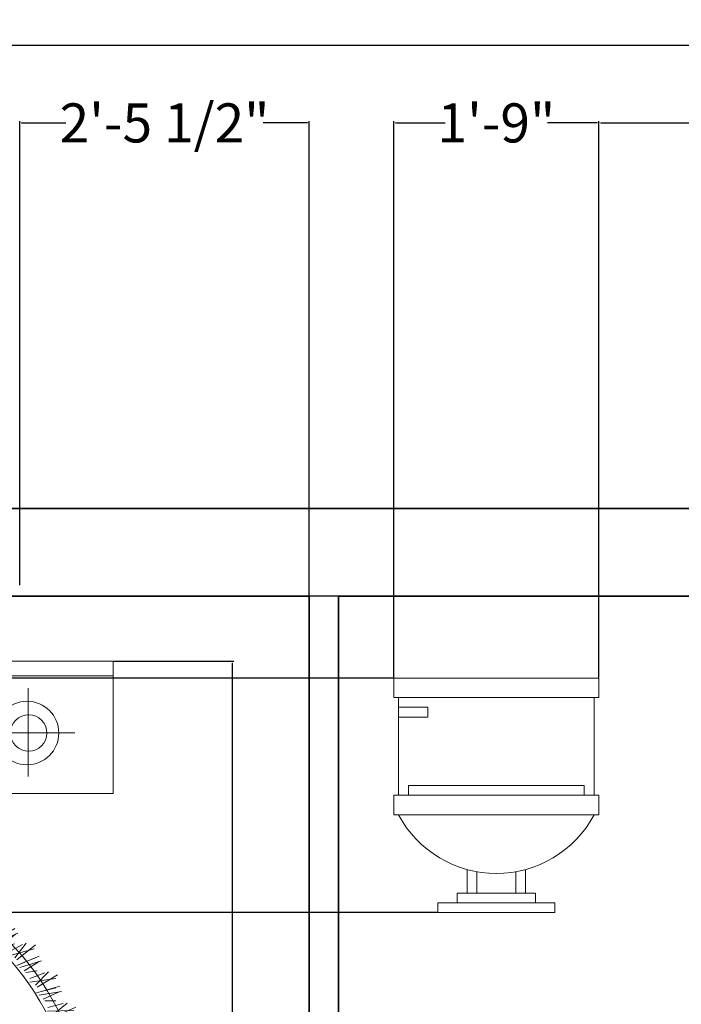
# Model space of a CAD drawing. Units: inches. Extents: x 311 to 754, y 60 to 497.
# Tile 5 of 11: x 462 to 530, y 396 to 497. Entities that reach past the tile are written whole.
import ezdxf

# ---------------------------------------------------------------- set-up
doc = ezdxf.new("R2010")
doc.units = ezdxf.units.IN
doc.header["$MEASUREMENT"] = 0
for name, color, linetype, lineweight in [('A-ANNO-DIMS', 2, 'Continuous', 18), ('A-FLOR-FIXT', 9, 'Continuous', 18), ('A-WALL', 7, 'Continuous', 35), ('beds', 70, 'Continuous', 13)]:
    doc.layers.add(name, color=color, linetype=linetype, lineweight=lineweight)
doc.styles.get("Standard").update_dxf_attribs({"font": 'arial.ttf'})
doc.dimstyles.get("Standard").update_dxf_attribs({"dimtxt": 4, "dimasz": 0.18, "dimexe": 0.18, "dimexo": 0.0625, "dimgap": 0.09, "dimtad": 0, "dimtih": 1, "dimtoh": 1, "dimdec": 0, "dimrnd": 6, "dimzin": 0, "dimdsep": 46, "dimlunit": 3, "dimtxsty": 'Standard', "dimcen": 0.09, "dimadec": 0, "dimazin": 0, "dimtfac": 1, "dimtdec": 0, "dimtofl": 0, "dimtmove": 0, "dimatfit": 3, "dimfxl": 1, "dimtolj": 1, "dimtzin": 0, "dimarcsym": 0})

# ---------------------------------------------------------------- blocks, each defined once
blk = doc.blocks.new('A$C57792D97')
for p, q in [((0.6, 2.6235), (0, 2.6235)), ((0, 2.6235), (0, 2.1735)), ((2.1, 2.6235), (0.6, 2.6235)), ((0.6, 2.6235), (0.6, 0.6235)), ((0.6, 0.6235), (0.6, 2.6235)), ((0.6, 2.1735), (0.6, 2.6235)), ((2.1, 0.6235), (2.1, 2.6235)), ((2.7, 2.6235), (2.1, 2.6235)), ((2.1, 2.6235), (2.1, 2.1735)), ((2.7, 2.1735), (2.7, 2.6235)), ((0.6, 2.5735), (0, 2.5735)), ((2.1, 2.5735), (0.6, 2.5735)), ((2.7, 2.5735), (2.1, 2.5735)), ((2.4103, 2.2312), (2.4103, 2.5317)), ((2.2593, 2.3802), (2.5698, 2.3802)), ((1.5491, 2.1955), (1.5516, 2.1955)), ((0, 2.1735), (0.6, 2.1735)), ((0.6, 2.1518), (0.8661, 2.1518)), ((2.1, 2.1735), (2.7, 2.1735)), ((0.6, 1.9518), (1.4767, 1.9518)), ((0.63, 0.6535), (0.63, 1.9518)), ((0.9906, 1.8942), (0.9508, 1.934)), ((1.4149, 1.8942), (1.3751, 1.934)), ((0.9906, 1.8942), (0.9344, 1.8942)), ((0.9906, 1.8942), (0.9508, 1.8544)), ((1.4149, 1.8942), (1.3586, 1.8942)), ((1.4149, 1.8942), (1.3751, 1.8544)), ((2.142, 1.8959), (2.1018, 1.8254)), ((2.1679, 1.8652), (2.1088, 1.8077)), ((2.1584, 1.8544), (2.1201, 1.8188)), ((2.1812, 1.8524), (2.1207, 1.8046)), ((2.1749, 1.8475), (2.1394, 1.7993)), ((2.1799, 1.8155), (2.1465, 1.7971)), ((2.2066, 1.8191), (2.1664, 1.7827)), ((2.249, 1.8154), (2.1711, 1.7709)), ((2.2173, 1.8274), (2.1931, 1.7688)), ((2.2496, 1.8292), (2.2008, 1.7642)), ((2.07, 1.7793), (2.07, 0.6535)), ((2.2713, 1.7954), (2.2055, 1.7458)), ((2.283, 1.7811), (2.2169, 1.7413)), ((2.2607, 1.7859), (2.2181, 1.7554)), ((2.2761, 1.777), (2.2348, 1.7337)), ((2.277, 1.7446), (2.2416, 1.7306)), ((2.304, 1.7449), (2.2596, 1.7138)), ((2.3157, 1.7518), (2.2843, 1.6966)), ((2.3479, 1.7495), (2.2914, 1.6911)), ((0.7785, 1.6821), (0.7387, 1.7219)), ((1.2027, 1.6821), (1.163, 1.7219)), ((1.627, 1.6821), (1.5872, 1.7219)), ((2.0513, 1.6821), (2.0115, 1.7219)), ((2.3456, 1.7359), (2.2627, 1.7015)), ((2.3653, 1.7133), (2.2937, 1.6723)), ((0.7785, 1.6821), (0.7222, 1.6821)), ((0.7785, 1.6821), (0.7387, 1.6423)), ((1.2027, 1.6821), (1.1465, 1.6821)), ((1.2027, 1.6821), (1.163, 1.6423)), ((1.627, 1.6821), (1.5708, 1.6821)), ((1.627, 1.6821), (1.5872, 1.6423)), ((2.0513, 1.6821), (1.995, 1.6821)), ((2.0513, 1.6821), (2.0115, 1.6423)), ((2.3751, 1.6976), (2.3045, 1.6664)), ((2.3535, 1.7051), (2.3075, 1.6802)), ((2.3677, 1.6944), (2.3213, 1.6565)), ((2.3645, 1.6621), (2.3277, 1.6526)), ((2.3913, 1.659), (2.3434, 1.6337)), ((2.4314, 1.6449), (2.3449, 1.6211)), ((2.4038, 1.6644), (2.3657, 1.6136)), ((2.4355, 1.6581), (2.372, 1.6073)), ((2.4482, 1.62), (2.372, 1.5882)), ((2.4354, 1.6134), (2.3867, 1.5944)), ((2.2754, 1.598), (2.2534, 1.5939)), ((2.2736, 1.5771), (2.2535, 1.594)), ((2.2736, 1.5771), (2.2754, 1.598)), ((2.4559, 1.6032), (2.382, 1.581)), ((2.4482, 1.6009), (2.3974, 1.5692)), ((2.3123, 1.541), (2.2911, 1.5481)), ((2.3006, 1.5236), (2.2912, 1.5481)), ((2.441, 1.5693), (2.4032, 1.5645)), ((2.4672, 1.5629), (2.4164, 1.5438)), ((2.5052, 1.5438), (2.4164, 1.5311)), ((2.4802, 1.5667), (2.4361, 1.5211)), ((2.5109, 1.5564), (2.4416, 1.514)), ((0.9906, 1.47), (0.9508, 1.5097)), ((1.4149, 1.47), (1.3751, 1.5097)), ((1.8391, 1.47), (1.7994, 1.5097)), ((2.3006, 1.5236), (2.3123, 1.541)), ((2.5187, 1.517), (2.4392, 1.4951)), ((2.5052, 1.5121), (2.4545, 1.4994)), ((2.5243, 1.4994), (2.4482, 1.4867)), ((2.5163, 1.4981), (2.462, 1.473)), ((0.9906, 1.47), (0.9344, 1.47)), ((0.9906, 1.47), (0.9508, 1.4302)), ((1.4149, 1.47), (1.3586, 1.47)), ((1.4149, 1.47), (1.3751, 1.4302)), ((1.8391, 1.47), (1.7829, 1.47)), ((1.8391, 1.47), (1.7994, 1.4302)), ((2.5052, 1.4677), (2.4672, 1.4677)), ((2.5304, 1.458), (2.4777, 1.4454)), ((2.5438, 1.4601), (2.4943, 1.4204)), ((2.573, 1.4461), (2.4989, 1.4127)), ((2.5658, 1.4343), (2.4761, 1.4328)), ((2.5758, 1.406), (2.4942, 1.3942)), ((2.5791, 1.3878), (2.502, 1.3848)), ((2.5618, 1.4028), (2.5099, 1.3966)), ((2.571, 1.3876), (2.514, 1.3695)), ((2.2534, 1.3469), (2.2315, 1.3429)), ((2.2516, 1.326), (2.2315, 1.3429)), ((2.2516, 1.326), (2.2535, 1.347)), ((2.5562, 1.3587), (2.5185, 1.3635)), ((2.58, 1.346), (2.5261, 1.3402)), ((2.5936, 1.3464), (2.5395, 1.3132)), ((2.1596, 1.3147), (2.1502, 1.3392)), ((2.1714, 1.3321), (2.1502, 1.3392)), ((2.1596, 1.3147), (2.1714, 1.3321)), ((2.3632, 1.3229), (2.33, 1.319)), ((2.3584, 1.2918), (2.33, 1.319)), ((2.3584, 1.2918), (2.3632, 1.3229)), ((2.6121, 1.3181), (2.523, 1.3279)), ((2.6207, 1.3289), (2.5431, 1.305)), ((0.7785, 1.2578), (0.7387, 1.2976)), ((1.2027, 1.2578), (1.163, 1.2976)), ((1.627, 1.2578), (1.5872, 1.2976)), ((2.0513, 1.2578), (2.0115, 1.2976)), ((2.6185, 1.2888), (2.5361, 1.2873)), ((2.6195, 1.2703), (2.5426, 1.277)), ((2.6042, 1.2873), (2.5519, 1.2877)), ((0.7785, 1.2578), (0.7222, 1.2578)), ((0.7785, 1.2578), (0.7387, 1.218)), ((1.2027, 1.2578), (1.1465, 1.2578)), ((1.2027, 1.2578), (1.163, 1.218)), ((1.627, 1.2578), (1.5708, 1.2578)), ((1.627, 1.2578), (1.5872, 1.218)), ((2.0513, 1.2578), (1.995, 1.2578)), ((2.0513, 1.2578), (2.0115, 1.218)), ((2.4134, 1.2295), (2.404, 1.254)), ((2.4252, 1.2469), (2.404, 1.254)), ((2.4134, 1.2295), (2.4252, 1.2469)), ((2.6115, 1.2711), (2.5526, 1.2603)), ((2.5932, 1.2443), (2.5563, 1.2538)), ((2.6435, 1.197), (2.5563, 1.2178)), ((2.6152, 1.2287), (2.561, 1.2296)), ((2.6287, 1.2274), (2.5709, 1.2013)), ((2.6462, 1.1671), (2.5642, 1.176)), ((2.6534, 1.2066), (2.5734, 1.1926)), ((2.6319, 1.1675), (2.58, 1.1743)), ((2.4947, 1.1445), (2.4728, 1.1404)), ((2.4929, 1.1236), (2.4728, 1.1404)), ((2.4929, 1.1236), (2.4948, 1.1445)), ((2.6449, 1.1486), (2.5694, 1.1649)), ((2.637, 1.1504), (2.5773, 1.147)), ((2.6155, 1.1261), (2.5801, 1.1402)), ((2.6353, 1.1079), (2.5817, 1.1156)), ((0.9906, 1.0457), (0.9508, 1.0855)), ((1.4149, 1.0457), (1.3751, 1.0855)), ((1.8391, 1.0457), (1.7994, 1.0855)), ((2.2315, 1.0959), (2.2095, 1.0919)), ((2.2297, 1.075), (2.2096, 1.0919)), ((2.2297, 1.075), (2.2315, 1.0959)), ((2.6595, 1.0729), (2.5756, 1.1045)), ((2.6486, 1.1049), (2.588, 1.0862)), ((2.6705, 1.0812), (2.5894, 1.0774)), ((0.9906, 1.0457), (0.9344, 1.0457)), ((0.9906, 1.0457), (0.9508, 1.0059)), ((1.4149, 1.0457), (1.3586, 1.0457)), ((1.4149, 1.0457), (1.3751, 1.0059)), ((1.8391, 1.0457), (1.7829, 1.0457)), ((1.8391, 1.0457), (1.7994, 1.0059)), ((2.2725, 1.0206), (2.2631, 1.0451)), ((2.2842, 1.038), (2.2631, 1.0451)), ((2.6584, 1.0429), (2.5782, 1.062)), ((2.6548, 1.0248), (2.582, 1.0503)), ((2.6442, 1.045), (2.5937, 1.0584)), ((2.2725, 1.0206), (2.2843, 1.038)), ((2.6472, 1.0275), (2.5875, 1.0316)), ((2.6228, 1.0061), (2.5895, 1.0244)), ((2.6598, 0.9477), (2.5805, 0.9897)), ((2.6402, 0.9855), (2.588, 0.9999)), ((2.653, 0.9809), (2.5905, 0.97)), ((2.3053, 0.9493), (2.272, 0.9455)), ((2.3005, 0.9182), (2.2721, 0.9455)), ((2.3005, 0.9182), (2.3053, 0.9494)), ((2.5263, 0.9355), (2.5169, 0.96)), ((2.538, 0.9528), (2.5169, 0.9599)), ((2.5263, 0.9355), (2.5381, 0.9529)), ((2.655, 0.9181), (2.5778, 0.9471)), ((2.6718, 0.9546), (2.5908, 0.961)), ((2.6412, 0.9221), (2.5927, 0.9416)), ((2.6491, 0.9006), (2.5801, 0.9351)), ((2.6419, 0.9043), (2.5832, 0.9159)), ((2.6151, 0.8861), (2.5843, 0.9085)), ((0.7785, 0.8336), (0.7387, 0.8733)), ((1.2027, 0.8336), (1.163, 0.8733)), ((1.627, 0.8336), (1.5872, 0.8733)), ((2.0513, 0.8336), (2.0115, 0.8733)), ((2.4728, 0.8934), (2.4508, 0.8894)), ((2.471, 0.8725), (2.4509, 0.8894)), ((2.471, 0.8725), (2.4728, 0.8934)), ((2.6444, 0.8236), (2.571, 0.8751)), ((2.6297, 0.8635), (2.5797, 0.8843)), ((2.2095, 0.8449), (2.1876, 0.8408)), ((2.2077, 0.824), (2.1876, 0.8408)), ((2.2077, 0.824), (2.2095, 0.8449)), ((2.6572, 0.8289), (2.5776, 0.8454)), ((2.6418, 0.8573), (2.5785, 0.8543)), ((0.7785, 0.8336), (0.7222, 0.8336)), ((0.7785, 0.8336), (0.7387, 0.7938)), ((1.2027, 0.8336), (1.1465, 0.8336)), ((1.2027, 0.8336), (1.163, 0.7938)), ((1.627, 0.8336), (1.5708, 0.8336)), ((1.627, 0.8336), (1.5872, 0.7938)), ((2.0513, 0.8336), (1.995, 0.8336)), ((2.0513, 0.8336), (2.0115, 0.7938)), ((2.1316, 0.8117), (2.1222, 0.8362)), ((2.1433, 0.8291), (2.1222, 0.8362)), ((2.1316, 0.8117), (2.1434, 0.8291)), ((2.6359, 0.7948), (2.5629, 0.8332)), ((2.6279, 0.7781), (2.5637, 0.821)), ((2.6227, 0.8004), (2.577, 0.8259)), ((1.9462, 0.7963), (1.9243, 0.7923)), ((2.6212, 0.7827), (2.5644, 0.8015)), ((2.5923, 0.768), (2.5646, 0.7941)), ((1.683, 0.7477), (1.661, 0.7437)), ((2.3854, 0.7265), (2.376, 0.751)), ((2.3971, 0.7439), (2.376, 0.751)), ((2.3854, 0.7265), (2.3972, 0.7439)), ((2.6136, 0.7023), (2.5472, 0.7626)), ((2.6153, 0.7361), (2.552, 0.7411)), ((2.604, 0.7437), (2.557, 0.7707)), ((2.5915, 0.6593), (2.5332, 0.7099)), ((2.6016, 0.6748), (2.534, 0.7221)), ((2.5892, 0.6821), (2.547, 0.7131)), ((2.6269, 0.706), (2.5501, 0.7323)), ((1.4197, 0.6992), (1.3978, 0.6951)), ((2.5549, 0.6537), (2.5307, 0.6831)), ((2.5855, 0.6646), (2.5315, 0.6905)), ((0.9906, 0.6214), (0.9508, 0.6612)), ((1.1564, 0.6506), (1.1345, 0.6466)), ((1.4149, 0.6214), (1.3751, 0.6612)), ((1.8391, 0.6214), (1.7994, 0.6612)), ((2.4508, 0.6424), (2.4289, 0.6383)), ((2.449, 0.6215), (2.4289, 0.6384)), ((2.449, 0.6215), (2.4508, 0.6424)), ((2.5678, 0.5858), (2.5095, 0.654)), ((2.5635, 0.6282), (2.5203, 0.6608)), ((2.02, 0.6035), (0.6716, 0.6035)), ((0.9906, 0.6214), (0.9344, 0.6214)), ((0.9906, 0.6214), (0.9727, 0.6035)), ((1.4149, 0.6214), (1.3586, 0.6214)), ((1.4149, 0.6214), (1.397, 0.6035)), ((1.8391, 0.6214), (1.7829, 0.6214)), ((1.8391, 0.6214), (1.8212, 0.6035)), ((2.5405, 0.546), (2.489, 0.6034)), ((2.5524, 0.5601), (2.4913, 0.6155)), ((2.541, 0.5688), (2.5031, 0.6049)), ((2.5815, 0.5878), (2.5085, 0.6236)), ((2.5737, 0.6192), (2.5116, 0.632)), ((0.6417, 0.5735), (2.05, 0.5735)), ((0.8932, 0.6021), (0.8712, 0.598)), ((1.3422, 0.5642), (1.3386, 0.5735)), ((1.3422, 0.5642), (1.3485, 0.5735)), ((2.1875, 0.5938), (2.1656, 0.5898)), ((2.1857, 0.5729), (2.1656, 0.5898)), ((2.1857, 0.5729), (2.1876, 0.5938)), ((2.2473, 0.5758), (2.2141, 0.5719)), ((2.2425, 0.5447), (2.2141, 0.572)), ((2.2425, 0.5447), (2.2474, 0.5758)), ((2.5035, 0.545), (2.4831, 0.5772)), ((2.5352, 0.552), (2.4849, 0.5844)), ((0.8142, 0.5177), (0.8685, 0.5428)), ((1.9243, 0.5453), (1.9023, 0.5412)), ((1.9225, 0.5244), (1.9024, 0.5412)), ((1.9225, 0.5244), (1.9243, 0.5453)), ((2.2445, 0.5176), (2.2351, 0.5421)), ((2.5078, 0.476), (2.4585, 0.551)), ((2.5088, 0.5186), (2.47, 0.5564)), ((0.8062, 0.5164), (0.8823, 0.5291)), ((0.8118, 0.4988), (0.8913, 0.5207)), ((0.8253, 0.5037), (0.876, 0.5164)), ((1.6077, 0.4964), (1.5865, 0.5035)), ((1.596, 0.479), (1.5866, 0.5035)), ((1.8485, 0.5294), (1.8152, 0.5255)), ((1.8437, 0.4983), (1.8153, 0.5256)), ((1.8437, 0.4983), (1.8485, 0.5294)), ((2.2445, 0.5176), (2.2562, 0.535)), ((2.4757, 0.4399), (2.4318, 0.5034)), ((2.4893, 0.4525), (2.4356, 0.515)), ((2.4791, 0.4625), (2.446, 0.503)), ((2.5216, 0.4763), (2.4537, 0.5209)), ((2.5178, 0.5084), (2.4578, 0.5289)), ((0.8196, 0.4594), (0.8889, 0.5018)), ((0.8253, 0.472), (0.9141, 0.4847)), ((0.8503, 0.4491), (0.8944, 0.4947)), ((0.8633, 0.4529), (0.9141, 0.472)), ((1.4496, 0.483), (1.4163, 0.4791)), ((1.4448, 0.4519), (1.4164, 0.4792)), ((1.4448, 0.4519), (1.4496, 0.483)), ((1.596, 0.479), (1.6077, 0.4964)), ((1.661, 0.4967), (1.6391, 0.4927)), ((1.6592, 0.4758), (1.6391, 0.4927)), ((1.6592, 0.4758), (1.661, 0.4967)), ((2.4389, 0.4436), (2.4227, 0.478)), ((2.4712, 0.4466), (2.4253, 0.485)), ((0.8823, 0.4149), (0.9331, 0.4466)), ((0.8895, 0.4465), (0.9273, 0.4513)), ((0.9592, 0.4578), (0.938, 0.4649)), ((0.9403, 0.459), (0.9381, 0.4649)), ((0.9508, 0.4454), (0.9592, 0.4578)), ((1.0507, 0.4366), (1.0175, 0.4327)), ((1.0459, 0.4055), (1.0507, 0.4366)), ((1.3977, 0.4481), (1.3758, 0.4441)), ((1.3959, 0.4272), (1.3758, 0.4441)), ((1.3959, 0.4272), (1.3978, 0.4482)), ((2.4345, 0.3746), (2.395, 0.4552)), ((2.4409, 0.4167), (2.4071, 0.4591)), ((0.8746, 0.4126), (0.9485, 0.4347)), ((0.8823, 0.3958), (0.9585, 0.4275)), ((0.895, 0.3577), (0.9585, 0.4085)), ((0.8951, 0.4024), (0.9438, 0.4214)), ((1.0459, 0.4055), (1.0175, 0.4328)), ((1.8615, 0.4113), (1.8403, 0.4184)), ((1.8498, 0.3939), (1.8404, 0.4184)), ((1.8498, 0.3939), (1.8615, 0.4113)), ((2.3981, 0.3428), (2.3625, 0.4113)), ((2.4132, 0.3535), (2.3678, 0.4224)), ((2.4043, 0.3648), (2.3766, 0.4092)), ((2.4482, 0.3731), (2.3865, 0.4259)), ((2.4485, 0.4055), (2.3915, 0.4334)), ((0.8991, 0.3709), (0.9856, 0.3946)), ((0.9267, 0.3514), (0.9648, 0.4022)), ((0.9392, 0.3568), (0.9872, 0.3821)), ((1.1345, 0.3996), (1.1125, 0.3955)), ((1.1327, 0.3787), (1.1126, 0.3955)), ((1.1327, 0.3787), (1.1345, 0.3996)), ((1.213, 0.3727), (1.1918, 0.3798)), ((1.2013, 0.3553), (1.1919, 0.3798)), ((1.2013, 0.3553), (1.213, 0.3727)), ((2.3607, 0.3242), (2.3324, 0.3704)), ((2.3621, 0.3511), (2.3503, 0.3873)), ((2.3945, 0.35), (2.3538, 0.3939)), ((0.9555, 0.3182), (1.026, 0.3494)), ((0.9628, 0.3214), (1.0092, 0.3592)), ((0.9652, 0.3025), (1.0368, 0.3435)), ((0.966, 0.3537), (1.0029, 0.3631)), ((0.977, 0.3107), (1.023, 0.3356)), ((2.1656, 0.3428), (2.1436, 0.3387)), ((2.1638, 0.3219), (2.1437, 0.3388)), ((2.1638, 0.3219), (2.1656, 0.3428)), ((2.3253, 0.265), (2.2888, 0.3389)), ((2.3625, 0.28), (2.3078, 0.3401)), ((2.3668, 0.3121), (2.3138, 0.3469)), ((2.3491, 0.2832), (2.32, 0.3681)), ((0.9826, 0.2663), (1.0392, 0.3246)), ((0.9849, 0.2799), (1.0678, 0.3143)), ((1.0148, 0.264), (1.0462, 0.3191)), ((1.0265, 0.2709), (1.0709, 0.302)), ((2.1153, 0.3261), (2.0941, 0.3332)), ((2.1036, 0.3087), (2.0942, 0.3332)), ((2.1036, 0.3087), (2.1153, 0.3261)), ((2.2743, 0.2689), (2.2671, 0.3063)), ((2.3063, 0.2638), (2.2714, 0.3124)), ((2.309, 0.2562), (2.2823, 0.3286)), ((2.3179, 0.2773), (2.2959, 0.3247)), ((1.0475, 0.2347), (1.1136, 0.2745)), ((1.0535, 0.2712), (1.0889, 0.2852)), ((1.0544, 0.2388), (1.0957, 0.2821)), ((1.0592, 0.2203), (1.125, 0.27)), ((1.4668, 0.2875), (1.4456, 0.2946)), ((1.4551, 0.2701), (1.4457, 0.2946)), ((1.4551, 0.2701), (1.4668, 0.2875)), ((1.9023, 0.2942), (1.8804, 0.2902)), ((1.9005, 0.2733), (1.8804, 0.2902)), ((1.9005, 0.2733), (1.9023, 0.2942)), ((2.2741, 0.2296), (2.2258, 0.2708)), ((2.2529, 0.2032), (2.2346, 0.291)), ((2.2695, 0.2424), (2.2473, 0.2918)), ((1.0699, 0.2299), (1.1124, 0.2604)), ((1.0809, 0.1866), (1.1297, 0.2516)), ((1.0815, 0.2004), (1.1594, 0.2449)), ((1.1132, 0.1884), (1.1374, 0.247)), ((1.639, 0.2457), (1.6171, 0.2416)), ((1.6372, 0.2248), (1.6171, 0.2416)), ((1.6372, 0.2248), (1.6391, 0.2457)), ((2.1768, 0.1984), (2.1745, 0.2364)), ((2.208, 0.1893), (2.1795, 0.2419)), ((2.2097, 0.1814), (2.1923, 0.2566)), ((2.227, 0.1881), (2.2001, 0.2661)), ((2.2212, 0.2012), (2.2053, 0.2511)), ((2.2658, 0.1984), (2.2191, 0.2649)), ((1.1239, 0.1967), (1.1641, 0.2331)), ((1.1493, 0.1634), (1.2098, 0.2112)), ((1.1507, 0.2003), (1.184, 0.2187)), ((1.1556, 0.1683), (1.1911, 0.2165)), ((1.1626, 0.1506), (1.2217, 0.2081)), ((1.7206, 0.2023), (1.6994, 0.2094)), ((1.7089, 0.1849), (1.6995, 0.2095)), ((1.7089, 0.1849), (1.7206, 0.2024)), ((2.1198, 0.1242), (2.1029, 0.2049)), ((2.1596, 0.1295), (2.1216, 0.2013)), ((2.1718, 0.1594), (2.129, 0.2063)), ((2.1474, 0.1359), (2.1403, 0.2253)), ((2.1688, 0.1727), (2.1529, 0.2245)), ((1.1721, 0.1614), (1.2104, 0.197)), ((1.1873, 0.1336), (1.259, 0.1875)), ((1.1885, 0.1199), (1.2287, 0.1904)), ((1.2203, 0.1256), (1.237, 0.1868)), ((1.2299, 0.1352), (1.2652, 0.1764)), ((1.3758, 0.1971), (1.3538, 0.193)), ((1.374, 0.1762), (1.3539, 0.1931)), ((1.374, 0.1762), (1.3758, 0.1971)), ((2.0343, 0.0824), (2.0385, 0.172)), ((2.0601, 0.1162), (2.0509, 0.1696)), ((2.0714, 0.1407), (2.0737, 0.1787)), ((2.1011, 0.1277), (2.0794, 0.1835)), ((2.1018, 0.1197), (2.0939, 0.1965)), ((2.1157, 0.1379), (2.1062, 0.1893)), ((1.2559, 0.1422), (1.2867, 0.1646)), ((1.2592, 0.1054), (1.3133, 0.1604)), ((1.2649, 0.111), (1.2941, 0.1633)), ((1.2741, 0.0944), (1.3255, 0.1588)), ((1.282, 0.1063), (1.3156, 0.1464)), ((1.3007, 0.0806), (1.3651, 0.1431)), ((1.3035, 0.0671), (1.3346, 0.1421)), ((1.3344, 0.0768), (1.3433, 0.1396)), ((1.7905, 0.1559), (1.7573, 0.152)), ((1.7857, 0.1248), (1.7573, 0.152)), ((1.7857, 0.1248), (1.7906, 0.1559)), ((1.9873, 0.08), (1.9728, 0.1381)), ((1.9871, 0.072), (1.9889, 0.1491)), ((2.0054, 0.0742), (1.9988, 0.1564)), ((2.0031, 0.0883), (2.0001, 0.1405)), ((2.0456, 0.0745), (2.0169, 0.1505)), ((2.0614, 0.1027), (2.0249, 0.1545)), ((1.3427, 0.0876), (1.3725, 0.1328)), ((1.3677, 0.0977), (1.3954, 0.1238)), ((1.3755, 0.0616), (1.4223, 0.1229)), ((1.3804, 0.0679), (1.4028, 0.1234)), ((1.3916, 0.0525), (1.4346, 0.1229)), ((1.3981, 0.0653), (1.4264, 0.1093)), ((1.4198, 0.0422), (1.4758, 0.1123)), ((1.4243, 0.0292), (1.4458, 0.1075)), ((1.4537, 0.0427), (1.4546, 0.1061)), ((1.4606, 0.0544), (1.4845, 0.103)), ((1.5135, 0.0258), (1.5473, 0.101)), ((1.7925, 0.0197), (1.8188, 0.1054)), ((1.8429, 0.0669), (1.8547, 0.1031)), ((1.8685, 0.047), (1.8614, 0.1064)), ((1.8672, 0.039), (1.8787, 0.1154)), ((1.8852, 0.0532), (1.8888, 0.1054)), ((1.8857, 0.0389), (1.8894, 0.1213)), ((1.9256, 0.0342), (1.9067, 0.1132)), ((1.9448, 0.0601), (1.9151, 0.1162)), ((1.9154, 0.0434), (1.9307, 0.1318)), ((1.9452, 0.0737), (1.9428, 0.1279)), ((1.9595, 0.0966), (1.9666, 0.134)), ((1.4841, 0.0676), (1.5083, 0.0969)), ((1.4964, 0.0327), (1.5351, 0.0995)), ((1.5005, 0.0397), (1.5158, 0.0975)), ((1.5183, 0.0393), (1.5409, 0.0865)), ((1.5428, 0.0191), (1.5896, 0.0956)), ((1.5489, 0.0067), (1.5603, 0.0871)), ((1.5763, 0.0238), (1.5693, 0.0868)), ((1.5817, 0.0362), (1.5994, 0.0875)), ((1.6034, 0.0523), (1.6237, 0.0845)), ((1.6199, 0.0192), (1.65, 0.0903)), ((1.6232, 0.0266), (1.631, 0.086)), ((1.6378, 0.0145), (1.6619, 0.0934)), ((1.6409, 0.0285), (1.6573, 0.0782)), ((1.6677, 0.0115), (1.7045, 0.0933)), ((1.6753, 0), (1.6766, 0.0812)), ((1.7004, 0.0204), (1.6855, 0.0821)), ((1.7041, 0.0334), (1.7152, 0.0865)), ((1.7236, 0.0521), (1.7398, 0.0865)), ((1.7442, 0.0214), (1.7651, 0.0956)), ((1.7465, 0.0291), (1.7469, 0.0889)), ((1.7625, 0.0189), (1.7765, 0.1002)), ((1.7638, 0.0332), (1.7739, 0.0845)), ((1.8015, 0.0092), (1.7926, 0.09)), ((1.8238, 0.0326), (1.8014, 0.0919)), ((1.8259, 0.046), (1.8303, 0.1))]:
    blk.add_line(p, q)
at = {"linetype": 'ByBlock'}
for p, q in [((0.3217, 2.5511), (0.3189, 2.5483)), ((0.3189, 2.5483), (0.3189, 2.3511)), ((0.5475, 2.5511), (0.3217, 2.5511)), ((0.5475, 2.5511), (0.5503, 2.5483)), ((0.5503, 2.5483), (0.5503, 2.3511)), ((0.3375, 2.5469), (0.3303, 2.5397)), ((0.3303, 2.5397), (0.3303, 2.3683)), ((0.3346, 2.5426), (0.3332, 2.5369)), ((0.3332, 2.5369), (0.3332, 2.4983)), ((0.3332, 2.5369), (0.346, 2.524)), ((0.3403, 2.5454), (0.3346, 2.5426)), ((0.3803, 2.5469), (0.3375, 2.5469)), ((0.3746, 2.5454), (0.3403, 2.5454)), ((0.3475, 2.5269), (0.3403, 2.5454)), ((0.346, 2.524), (0.3475, 2.5269)), ((0.346, 2.4597), (0.346, 2.524)), ((0.3475, 2.5269), (0.3675, 2.5269)), ((0.3675, 2.5269), (0.3746, 2.5454)), ((0.3689, 2.524), (0.3675, 2.5269)), ((0.3818, 2.5369), (0.3689, 2.524)), ((0.3689, 2.4597), (0.3689, 2.524)), ((0.3746, 2.5454), (0.3803, 2.5426)), ((0.386, 2.5397), (0.3803, 2.5469)), ((0.3803, 2.5426), (0.3818, 2.5369)), ((0.3818, 2.5369), (0.3818, 2.4983)), ((0.386, 2.3668), (0.386, 2.5397)), ((0.3989, 2.4597), (0.3989, 2.5354)), ((0.3989, 2.5354), (0.5418, 2.5354)), ((0.5418, 2.5354), (0.5418, 2.4597)), ((0.3332, 2.4983), (0.336, 2.4911)), ((0.336, 2.4911), (0.3403, 2.484)), ((0.3403, 2.484), (0.3417, 2.474)), ((0.3746, 2.484), (0.3732, 2.474)), ((0.3789, 2.4911), (0.3746, 2.484)), ((0.3818, 2.4983), (0.3789, 2.4911)), ((0.3417, 2.474), (0.3417, 2.4597)), ((0.3417, 2.4326), (0.3417, 2.4597)), ((0.346, 2.4597), (0.346, 2.3826)), ((0.3689, 2.4597), (0.3689, 2.3826)), ((0.3732, 2.474), (0.3732, 2.4597)), ((0.3732, 2.4326), (0.3732, 2.4597)), ((0.5418, 2.4597), (0.3989, 2.4597)), ((0.3989, 2.4426), (0.3989, 2.4568)), ((0.3989, 2.4568), (0.5361, 2.4568)), ((0.4675, 2.4568), (0.4675, 2.4426)), ((0.4789, 2.4568), (0.4789, 2.4426)), ((0.4903, 2.4568), (0.4903, 2.4426)), ((0.5018, 2.4568), (0.5018, 2.4426)), ((0.5132, 2.4568), (0.5132, 2.4426)), ((0.5246, 2.4568), (0.5246, 2.4426)), ((0.5361, 2.4568), (0.5361, 2.4426)), ((0.3332, 2.4083), (0.336, 2.4154)), ((0.336, 2.4154), (0.3403, 2.4226)), ((0.3403, 2.4226), (0.3417, 2.4326)), ((0.3746, 2.4226), (0.3732, 2.4326)), ((0.3789, 2.4154), (0.3746, 2.4226)), ((0.3818, 2.4083), (0.3789, 2.4154)), ((0.5361, 2.4426), (0.3989, 2.4426)), ((0.3989, 2.4197), (0.3989, 2.4111)), ((0.4103, 2.4197), (0.3989, 2.4197)), ((0.4103, 2.4111), (0.4103, 2.4197)), ((0.4275, 2.4197), (0.416, 2.4197)), ((0.416, 2.4197), (0.416, 2.4111)), ((0.4275, 2.4111), (0.4275, 2.4197)), ((0.4332, 2.4197), (0.4332, 2.4111)), ((0.4446, 2.4197), (0.4332, 2.4197)), ((0.4446, 2.4111), (0.4446, 2.4197)), ((0.4575, 2.4011), (0.4575, 2.4268)), ((0.4575, 2.4268), (0.5418, 2.4268)), ((0.4718, 2.424), (0.4761, 2.424)), ((0.4718, 2.4197), (0.4718, 2.424)), ((0.4761, 2.4197), (0.4718, 2.4197)), ((0.4761, 2.424), (0.4761, 2.4197)), ((0.4975, 2.424), (0.5018, 2.424)), ((0.4975, 2.4197), (0.4975, 2.424)), ((0.5018, 2.4197), (0.4975, 2.4197)), ((0.5018, 2.424), (0.5018, 2.4197)), ((0.5232, 2.4197), (0.5232, 2.424)), ((0.5232, 2.424), (0.5275, 2.424)), ((0.5275, 2.4197), (0.5232, 2.4197)), ((0.5275, 2.424), (0.5275, 2.4197)), ((0.5418, 2.4268), (0.5418, 2.4011)), ((0.3332, 2.3697), (0.3332, 2.4083)), ((0.3332, 2.3697), (0.346, 2.3826)), ((0.3475, 2.3797), (0.3403, 2.3611)), ((0.346, 2.3826), (0.3475, 2.3797)), ((0.3475, 2.3797), (0.3675, 2.3797)), ((0.3689, 2.3826), (0.3675, 2.3797)), ((0.3675, 2.3797), (0.3746, 2.3611)), ((0.3818, 2.3697), (0.3689, 2.3826)), ((0.3818, 2.3697), (0.3818, 2.4083)), ((0.3989, 2.4111), (0.4103, 2.4111)), ((0.3989, 2.404), (0.3989, 2.3954)), ((0.4103, 2.404), (0.3989, 2.404)), ((0.3989, 2.3954), (0.4103, 2.3954)), ((0.4103, 2.3883), (0.3989, 2.3883)), ((0.3989, 2.3883), (0.3989, 2.3797)), ((0.3989, 2.3797), (0.4103, 2.3797)), ((0.4103, 2.3954), (0.4103, 2.404)), ((0.4103, 2.3797), (0.4103, 2.3883)), ((0.416, 2.4111), (0.4275, 2.4111)), ((0.416, 2.404), (0.416, 2.3954)), ((0.4275, 2.404), (0.416, 2.404)), ((0.416, 2.3954), (0.4275, 2.3954)), ((0.4275, 2.3868), (0.416, 2.3868)), ((0.416, 2.3868), (0.416, 2.3783)), ((0.4275, 2.3954), (0.4275, 2.404)), ((0.4275, 2.3783), (0.4275, 2.3868)), ((0.4332, 2.4111), (0.4446, 2.4111)), ((0.4332, 2.404), (0.4332, 2.3954)), ((0.4446, 2.404), (0.4332, 2.404)), ((0.4332, 2.3954), (0.4446, 2.3954)), ((0.4446, 2.3868), (0.4332, 2.3868)), ((0.4332, 2.3868), (0.4332, 2.3783)), ((0.4446, 2.3954), (0.4446, 2.404)), ((0.4446, 2.3783), (0.4446, 2.3868)), ((0.5418, 2.4011), (0.4575, 2.4011)), ((0.4661, 2.394), (0.4803, 2.394)), ((0.4661, 2.3883), (0.4661, 2.394)), ((0.4803, 2.3883), (0.4661, 2.3883)), ((0.4718, 2.4083), (0.4761, 2.4083)), ((0.4718, 2.404), (0.4718, 2.4083)), ((0.4761, 2.404), (0.4718, 2.404)), ((0.4761, 2.4083), (0.4761, 2.404)), ((0.4803, 2.394), (0.4803, 2.3883)), ((0.4861, 2.3883), (0.4861, 2.394)), ((0.4861, 2.394), (0.5003, 2.394)), ((0.5003, 2.3883), (0.4861, 2.3883)), ((0.4975, 2.4083), (0.5018, 2.4083)), ((0.4975, 2.404), (0.4975, 2.4083)), ((0.5018, 2.404), (0.4975, 2.404)), ((0.5003, 2.394), (0.5003, 2.3883)), ((0.5018, 2.4083), (0.5018, 2.404)), ((0.5061, 2.3883), (0.5061, 2.394)), ((0.5061, 2.394), (0.5203, 2.394)), ((0.5203, 2.3883), (0.5061, 2.3883)), ((0.5203, 2.394), (0.5203, 2.3883)), ((0.5232, 2.4083), (0.5275, 2.4083)), ((0.5232, 2.404), (0.5232, 2.4083)), ((0.5275, 2.404), (0.5232, 2.404)), ((0.5261, 2.3883), (0.5261, 2.394)), ((0.5261, 2.394), (0.5403, 2.394)), ((0.5403, 2.3883), (0.5261, 2.3883)), ((0.5275, 2.4083), (0.5275, 2.404)), ((0.5403, 2.394), (0.5403, 2.3883)), ((0.2937, 2.3497), (0.2748, 2.3336)), ((0.2789, 2.3502), (0.2854, 2.3565)), ((0.2804, 2.3412), (0.2789, 2.3502)), ((0.2854, 2.3565), (0.2932, 2.3525)), ((0.2902, 2.3608), (0.294, 2.3648)), ((0.2932, 2.3525), (0.2902, 2.3608)), ((0.3053, 2.3601), (0.2937, 2.3497)), ((0.294, 2.3648), (0.2975, 2.3621)), ((0.2955, 2.3663), (0.298, 2.3689)), ((0.2975, 2.3621), (0.2955, 2.3663)), ((0.298, 2.3689), (0.3033, 2.3669)), ((0.3053, 2.3628), (0.3023, 2.3631)), ((0.3023, 2.3631), (0.3053, 2.3601)), ((0.3033, 2.3669), (0.3063, 2.3696)), ((0.3068, 2.3648), (0.3053, 2.3628)), ((0.3063, 2.3696), (0.3103, 2.3737)), ((0.3126, 2.3694), (0.3068, 2.3648)), ((0.3103, 2.3737), (0.3189, 2.3768)), ((0.3189, 2.3711), (0.3126, 2.3694)), ((0.3189, 2.3511), (0.3217, 2.3483)), ((0.3217, 2.3483), (0.3525, 2.3483)), ((0.3303, 2.3683), (0.3375, 2.3597)), ((0.3346, 2.364), (0.3332, 2.3697)), ((0.3403, 2.3611), (0.3346, 2.364)), ((0.3375, 2.3597), (0.3542, 2.3597)), ((0.3543, 2.3611), (0.3403, 2.3611)), ((0.3518, 2.3447), (0.3538, 2.354)), ((0.3538, 2.354), (0.3546, 2.3654)), ((0.3546, 2.3654), (0.3589, 2.3654)), ((0.3587, 2.3531), (0.3552, 2.3386)), ((0.3575, 2.3483), (0.5475, 2.3483)), ((0.3589, 2.3654), (0.3587, 2.3531)), ((0.3746, 2.3611), (0.3588, 2.3611)), ((0.3588, 2.3597), (0.3789, 2.3597)), ((0.3746, 2.3611), (0.3803, 2.364)), ((0.3789, 2.3597), (0.386, 2.3668)), ((0.3803, 2.364), (0.3818, 2.3697)), ((0.4103, 2.3711), (0.3989, 2.3711)), ((0.3989, 2.3711), (0.3989, 2.3626)), ((0.3989, 2.3626), (0.4103, 2.3626)), ((0.4103, 2.3626), (0.4103, 2.3711)), ((0.416, 2.3783), (0.4275, 2.3783)), ((0.416, 2.3711), (0.416, 2.3626)), ((0.4275, 2.3711), (0.416, 2.3711)), ((0.416, 2.3626), (0.4275, 2.3626)), ((0.4275, 2.3626), (0.4275, 2.3711)), ((0.4332, 2.3783), (0.4446, 2.3783)), ((0.4332, 2.3711), (0.4332, 2.3626)), ((0.4446, 2.3711), (0.4332, 2.3711)), ((0.4332, 2.3626), (0.4446, 2.3626)), ((0.4446, 2.3626), (0.4446, 2.3711)), ((0.4661, 2.3726), (0.4661, 2.364)), ((0.4803, 2.3726), (0.4661, 2.3726)), ((0.4661, 2.364), (0.4803, 2.364)), ((0.4803, 2.364), (0.4803, 2.3726)), ((0.5003, 2.3726), (0.4861, 2.3726)), ((0.4861, 2.3726), (0.4861, 2.364)), ((0.4861, 2.364), (0.5003, 2.364)), ((0.5003, 2.364), (0.5003, 2.3726)), ((0.5203, 2.3726), (0.5061, 2.3726)), ((0.5061, 2.3726), (0.5061, 2.364)), ((0.5061, 2.364), (0.5203, 2.364)), ((0.5203, 2.364), (0.5203, 2.3726)), ((0.5403, 2.3726), (0.5261, 2.3726)), ((0.5261, 2.3726), (0.5261, 2.364)), ((0.5261, 2.364), (0.5403, 2.364)), ((0.5403, 2.364), (0.5403, 2.3726)), ((0.5503, 2.3511), (0.5475, 2.3483)), ((0.2563, 2.3158), (0.2584, 2.3224)), ((0.2624, 2.31), (0.2563, 2.3158)), ((0.2584, 2.3224), (0.2676, 2.3221)), ((0.2592, 2.3253), (0.2618, 2.334)), ((0.2676, 2.3221), (0.2592, 2.3253)), ((0.2618, 2.334), (0.2705, 2.3331)), ((0.2746, 2.3331), (0.265, 2.3059)), ((0.2683, 2.3394), (0.2738, 2.3452)), ((0.2706, 2.3331), (0.2683, 2.3394)), ((0.2738, 2.3452), (0.2804, 2.3412)), ((0.3425, 2.3129), (0.3477, 2.3166)), ((0.3437, 2.3062), (0.3425, 2.3129)), ((0.3474, 2.3242), (0.3483, 2.3311)), ((0.3477, 2.3166), (0.3474, 2.3242)), ((0.3483, 2.3311), (0.3518, 2.3447)), ((0.352, 2.3175), (0.3512, 2.3158)), ((0.3512, 2.3158), (0.3544, 2.3126)), ((0.3552, 2.3386), (0.3518, 2.325)), ((0.3518, 2.325), (0.352, 2.3175)), ((0.2532, 2.3027), (0.2546, 2.31)), ((0.2621, 2.3001), (0.2532, 2.3027)), ((0.2546, 2.31), (0.2624, 2.31)), ((0.2546, 2.2958), (0.2621, 2.3001)), ((0.2558, 2.29), (0.2546, 2.2958)), ((0.2647, 2.2903), (0.2558, 2.29)), ((0.2578, 2.2825), (0.2647, 2.2903)), ((0.2601, 2.2767), (0.2578, 2.2825)), ((0.2685, 2.2793), (0.2601, 2.2767)), ((0.2644, 2.2715), (0.2685, 2.2793)), ((0.265, 2.3059), (0.2691, 2.2842)), ((0.2691, 2.2842), (0.2818, 2.2718)), ((0.3312, 2.2741), (0.3422, 2.288)), ((0.3492, 2.2776), (0.3405, 2.2793)), ((0.3405, 2.2793), (0.3445, 2.2712)), ((0.3422, 2.288), (0.3437, 2.3062)), ((0.3541, 2.2915), (0.3448, 2.2906)), ((0.3448, 2.2906), (0.3529, 2.2842)), ((0.3549, 2.3056), (0.3466, 2.3042)), ((0.3466, 2.3042), (0.3546, 2.2993)), ((0.3529, 2.2842), (0.3492, 2.2776)), ((0.3546, 2.2993), (0.3541, 2.2915)), ((0.3544, 2.3126), (0.3549, 2.3056)), ((0.2682, 2.268), (0.2644, 2.2715)), ((0.2763, 2.2715), (0.2682, 2.268)), ((0.2728, 2.2637), (0.2763, 2.2715)), ((0.2774, 2.2596), (0.2728, 2.2637)), ((0.2835, 2.2672), (0.2774, 2.2596)), ((0.2818, 2.2718), (0.2986, 2.2646)), ((0.2827, 2.2585), (0.2835, 2.2672)), ((0.2873, 2.2562), (0.2827, 2.2585)), ((0.2939, 2.262), (0.2873, 2.2562)), ((0.2942, 2.2541), (0.2939, 2.262)), ((0.2997, 2.2527), (0.2942, 2.2541)), ((0.2986, 2.2646), (0.3159, 2.266)), ((0.3029, 2.262), (0.2997, 2.2527)), ((0.3049, 2.2536), (0.3029, 2.262)), ((0.3098, 2.2541), (0.3049, 2.2536)), ((0.3133, 2.262), (0.3098, 2.2541)), ((0.3171, 2.2541), (0.3133, 2.262)), ((0.3159, 2.266), (0.3312, 2.2741)), ((0.3231, 2.2559), (0.3171, 2.2541)), ((0.3292, 2.2596), (0.3223, 2.2654)), ((0.3223, 2.2654), (0.3231, 2.2559)), ((0.3347, 2.2631), (0.3292, 2.2596)), ((0.3402, 2.266), (0.3335, 2.2709)), ((0.3335, 2.2709), (0.3347, 2.2631)), ((0.3445, 2.2712), (0.3402, 2.266))]:
    blk.add_line(p, q, dxfattribs=at)
for centre, radius in [((2.4068, 2.3792), 0.1082), ((2.4128, 2.3792), 0.062)]:
    blk.add_circle(centre, radius)
for centre, radius, start, end in [((0.8117, 1.4495), 1.1155, 75.3755, 98.4519), ((0.7133, 2.123), 0.4349, 62.6153, 98.6623), ((0.9995, 2.5566), 0.3518, 180.6066, 203.849), ((1.2711, 1.6927), 0.8548, 85.0132, 101.9962), ((1.5803, 0.4369), 2.1259, 84.0997, 95.547), ((7.229, 2.8402), 5.8612, 182.80995, 184.16642), ((1.505, 1.754), 0.7941, 71.9705, 99.0452), ((2.0384, 6.4739), 3.9297, 266.5056, 270.1818), ((0.9942, 1.5092), 1.0245, 76.8495, 84.445), ((-2.6554, 2.4937), 4.0011, 355.9906, 0.7251), ((1.6997, 1.5092), 1.0245, 76.8495, 84.445), ((2.5231, 2.3654), 0.505, 159.2551, 197.4606), ((6.5168, 1.1676), 5.2262, 165.6998, 168.4122), ((1.7461, 2.3905), 1.0686, 178.7205, 189.3246), ((2.4516, 2.3905), 1.0686, 178.7205, 189.3246), ((1.0382, 2.187), 0.3479, 146.8128, 174.9884), ((1.3553, 2.3447), 0.1322, 217.4973, 261.5591), ((2.6076, 3.8927), 1.7717, 246.8027, 251.3608), ((0.9964, 4.7934), 2.5939, 263.2521, 270.4789), ((1.1218, 3.4256), 1.2305, 265.1643, 280.0187), ((1.5587, 3.1365), 0.9332, 260.0314, 280.1788), ((1.8907, 2.8521), 0.6558, 255.2386, 283.2855), ((1.0153, 0.392), 1.7661, 72.4208, 94.846), ((0.7898, 0.8867), 1.2674, 53.0057, 86.5496), ((2.0108, 3.233), 1.2462, 248.2311, 274.1028), ((1.991, 2.6169), 0.8413, 238.5747, 277.4412), ((1.6653, 1.0079), 0.9493, 207.2312, 62.7432), ((1.6653, 1.0079), 0.9093, 208.5361, 61.4369), ((0.6787, 0.6517), 0.0487, 177.8916, 261.664), ((2.02, 0.6535), 0.05, 270, 0), ((0.6518, 0.6244), 0.0518, 180.9151, 258.7324), ((2.05, 0.6235), 0.05, 270, 0)]:
    blk.add_arc(centre, radius, start, end)
blk = doc.blocks.new('*U102')
for p, q in [((-10, 22), (-10, 12)), ((10, 12), (10, 22)), ((-10, 21), (-7, 21)), ((-7, 21), (-7, 20)), ((-7, 20), (-10, 20)), ((9, 13), (-9, 13)), ((-9, 13), (-9, 12)), ((9, 12), (9, 13)), ((10.5, 12), (-10.5, 12)), ((-10.5, 10), (-10.5, 12)), ((10.5, 12), (10.5, 10)), ((10.5, 10), (-10.5, 10)), ((-3, 4.4065), (-3, 2)), ((-2, 2), (-2, 4.1658)), ((2, 4.1658), (2, 2)), ((3, 2), (3, 4.4065)), ((4, 2), (-4, 2)), ((-4, 2), (-4, 1)), ((4, 1), (4, 2))]:
    blk.add_line(p, q)
for points in [[(10.5, 22), (10.5, 24), (-10.5, 24), (-10.5, 22)], [(6, 0), (6, 1), (-6, 1), (-6, 0)]]:
    blk.add_lwpolyline(points, close=True)
blk.add_arc((0, 15.3333), 11.3333, 208.0725, 331.9275)
blk = doc.blocks.new('*D103')
at = {"layer": 'A-ANNO-DIMS', "color": 0, "lineweight": -2, "transparency": 16777216}
for p, q in [((362.8, 447.3), (362.8, 494.8)), ((722.8, 447.3), (722.8, 494.8)), ((362.98, 494.62), (539.32, 494.62)), ((722.62, 494.62), (546.29, 494.62))]:
    blk.add_line(p, q, dxfattribs=at)
at = {"layer": 'A-ANNO-DIMS', "color": 0, "transparency": 16777216}
for points in [[(362.98, 494.65), (362.98, 494.59), (362.8, 494.62)], [(722.62, 494.65), (722.62, 494.59), (722.8, 494.62)]]:
    blk.add_solid(points, dxfattribs=at)
at = {"layer": 'Defpoints', "color": 0, "transparency": 16777216}
for p in [(722.8, 494.62), (362.8, 447.24), (722.8, 447.24)]:
    blk.add_point(p, dxfattribs=at)
at = {"layer": 'A-ANNO-DIMS', "color": 0, "transparency": 16777216, "insert": (542.8, 494.62), "char_height": 4, "attachment_point": 5}
blk.add_mtext("\\A1;30'", dxfattribs=at)
blk = doc.blocks.new('*D111')
at = {"layer": 'A-ANNO-DIMS', "color": 0, "lineweight": -2, "transparency": 16777216}
for p, q in [((471.79, 431.59), (484.09, 431.59)), ((483.91, 431.41), (483.91, 394.29)), ((483.91, 352.91), (483.91, 390.03)), ((471.79, 352.73), (484.09, 352.73))]:
    blk.add_line(p, q, dxfattribs=at)
at = {"layer": 'A-ANNO-DIMS', "color": 0, "transparency": 16777216}
for points in [[(483.88, 431.41), (483.94, 431.41), (483.91, 431.59)], [(483.88, 352.91), (483.94, 352.91), (483.91, 352.73)]]:
    blk.add_solid(points, dxfattribs=at)
at = {"layer": 'Defpoints', "color": 0, "transparency": 16777216}
for p in [(471.73, 431.59), (483.91, 431.59), (471.73, 352.73)]:
    blk.add_point(p, dxfattribs=at)
at = {"layer": 'A-ANNO-DIMS', "color": 0, "transparency": 16777216, "insert": (483.91, 392.16), "char_height": 4, "attachment_point": 5}
blk.add_mtext('\\A1;6\'-7" TYP.', dxfattribs=at)
blk = doc.blocks.new('*D119')
at = {"layer": 'A-ANNO-DIMS', "color": 0, "lineweight": -2, "transparency": 16777216}
for p, q in [((462.17, 439.39), (462.17, 486.86)), ((462.35, 486.68), (466.89, 486.68)), ((491.62, 486.68), (487.09, 486.68)), ((491.8, 438.3), (491.8, 486.86))]:
    blk.add_line(p, q, dxfattribs=at)
at = {"layer": 'A-ANNO-DIMS', "color": 0, "transparency": 16777216}
for points in [[(462.35, 486.71), (462.35, 486.65), (462.17, 486.68)], [(491.62, 486.71), (491.62, 486.65), (491.8, 486.68)]]:
    blk.add_solid(points, dxfattribs=at)
at = {"layer": 'Defpoints', "color": 0, "transparency": 16777216}
for p in [(491.8, 486.68), (462.17, 439.33), (491.8, 438.24)]:
    blk.add_point(p, dxfattribs=at)
at = {"layer": 'A-ANNO-DIMS', "color": 0, "transparency": 16777216, "insert": (476.99, 486.68), "char_height": 4, "attachment_point": 5}
blk.add_mtext('\\A1;2\'-5 1/2"', dxfattribs=at)
blk = doc.blocks.new('*D144')
at = {"layer": 'A-ANNO-DIMS', "color": 0, "lineweight": -2, "transparency": 16777216}
for p, q in [((500.44, 429.94), (500.44, 486.86)), ((500.62, 486.68), (505.72, 486.68)), ((521.26, 486.68), (516.16, 486.68)), ((521.44, 429.94), (521.44, 486.86))]:
    blk.add_line(p, q, dxfattribs=at)
at = {"layer": 'A-ANNO-DIMS', "color": 0, "transparency": 16777216}
for points in [[(500.62, 486.71), (500.62, 486.65), (500.44, 486.68)], [(521.26, 486.71), (521.26, 486.65), (521.44, 486.68)]]:
    blk.add_solid(points, dxfattribs=at)
at = {"layer": 'Defpoints', "color": 0, "transparency": 16777216}
for p in [(500.44, 486.68), (500.44, 429.88), (521.44, 429.88)]:
    blk.add_point(p, dxfattribs=at)
at = {"layer": 'A-ANNO-DIMS', "color": 0, "transparency": 16777216, "insert": (510.94, 486.68), "char_height": 4, "attachment_point": 5}
blk.add_mtext('\\A1;1\'-9"', dxfattribs=at)
blk = doc.blocks.new('*D145')
at = {"layer": 'A-ANNO-DIMS', "color": 0, "lineweight": -2, "transparency": 16777216}
for p, q in [((500.37, 429.88), (341.82, 429.88)), ((342, 429.7), (342, 420.01)), ((342, 406.06), (342, 415.74)), ((504.87, 405.88), (341.82, 405.88))]:
    blk.add_line(p, q, dxfattribs=at)
at = {"layer": 'A-ANNO-DIMS', "color": 0, "transparency": 16777216}
for points in [[(341.97, 429.7), (342.03, 429.7), (342, 429.88)], [(341.97, 406.06), (342.03, 406.06), (342, 405.88)]]:
    blk.add_solid(points, dxfattribs=at)
at = {"layer": 'Defpoints', "color": 0, "transparency": 16777216}
for p in [(342, 429.88), (500.44, 429.88), (504.94, 405.88)]:
    blk.add_point(p, dxfattribs=at)
at = {"layer": 'A-ANNO-DIMS', "color": 0, "transparency": 16777216, "insert": (342, 417.88), "char_height": 4, "attachment_point": 5}
blk.add_mtext('\\A1;2\'-0"', dxfattribs=at)
blk = doc.blocks.new('*D150')
at = {"layer": 'A-ANNO-DIMS', "color": 0, "lineweight": -2, "transparency": 16777216}
for p, q in [((521.44, 429.94), (521.44, 486.86)), ((521.62, 486.68), (532.86, 486.68)), ((533.04, 431.2), (533.04, 486.86)), ((533.04, 486.68), (533.22, 486.68))]:
    blk.add_line(p, q, dxfattribs=at)
at = {"layer": 'A-ANNO-DIMS', "color": 0, "transparency": 16777216}
for points in [[(521.62, 486.71), (521.62, 486.65), (521.44, 486.68)], [(532.86, 486.71), (532.86, 486.65), (533.04, 486.68)]]:
    blk.add_solid(points, dxfattribs=at)
at = {"layer": 'Defpoints', "color": 0, "transparency": 16777216}
for p in [(533.04, 486.68), (533.04, 431.14), (521.44, 429.88)]:
    blk.add_point(p, dxfattribs=at)
at = {"layer": 'A-ANNO-DIMS', "color": 0, "transparency": 16777216, "insert": (544.84, 486.68), "char_height": 4, "attachment_point": 5}
blk.add_mtext('\\A1;0\'-11 1/2"', dxfattribs=at)
blk = doc.blocks.new('*D151')
at = {"layer": 'A-ANNO-DIMS', "color": 0, "lineweight": -2, "transparency": 16777216}
for p, q in [((494.74, 438.24), (341.82, 438.24)), ((342, 438.06), (342, 436.22)), ((342, 430.06), (342, 431.9)), ((500.37, 429.88), (341.82, 429.88))]:
    blk.add_line(p, q, dxfattribs=at)
at = {"layer": 'A-ANNO-DIMS', "color": 0, "transparency": 16777216}
for points in [[(341.97, 438.06), (342.03, 438.06), (342, 438.24)], [(341.97, 430.06), (342.03, 430.06), (342, 429.88)]]:
    blk.add_solid(points, dxfattribs=at)
at = {"layer": 'Defpoints', "color": 0, "transparency": 16777216}
for p in [(494.8, 438.24), (342, 429.88), (500.44, 429.88)]:
    blk.add_point(p, dxfattribs=at)
at = {"layer": 'A-ANNO-DIMS', "color": 0, "transparency": 16777216, "insert": (342, 434.06), "char_height": 4, "attachment_point": 5}
blk.add_mtext('\\A1;0\'-8 1/2"', dxfattribs=at)

msp = doc.modelspace()

# ---------------------------------------------------------------- linework, layer by layer
at = {"layer": 'A-WALL'}
for p, q in [((722.8, 447.24), (362.8, 447.24)), ((491.8, 438.24), (371.8, 438.24)), ((491.8, 438.24), (491.8, 332.1)), ((494.8, 438.24), (494.8, 342.24)), ((563.8, 438.24), (494.8, 438.24))]:
    msp.add_line(p, q, dxfattribs=at)

# ---------------------------------------------------------------- block references
at = {"layer": 'A-FLOR-FIXT'}
msp.add_blockref('*U102', (510.94, 405.88), dxfattribs=at)
at = {"layer": 'beds', "xscale": 30.06046351726443, "yscale": 30.06046351726443, "zscale": 30.06046351726443}
msp.add_blockref('A$C57792D97', (390.57, 352.73), dxfattribs=at)

# ---------------------------------------------------------------- dimensions: what is measured, and where the dimension line sits
at = {"layer": 'A-ANNO-DIMS'}
for base, p1, p2, override, picture, middle in [((722.8, 494.62), (362.8, 447.24), (722.8, 447.24), {"dimclrd": 0, "dimclre": 0, "dimclrt": 0}, '*D103', (542.8, 494.62)), ((491.8, 486.68), (462.17, 439.33), (491.8, 438.24), {"dimdec": 1, "dimlfac": 1, "dimrnd": 0, "dimzin": 1, "dimdsep": 46, "dimlunit": 4, "dimfrac": 2}, '*D119', (476.99, 486.68)), ((533.04, 486.68), (521.44, 429.88), (533.04, 431.14), {"dimdec": 1, "dimlfac": 1, "dimrnd": 0, "dimzin": 1, "dimdsep": 46, "dimlunit": 4, "dimfrac": 2}, '*D150', (544.84, 486.68)), ((500.44, 486.68), (521.44, 429.88), (500.44, 429.88), {"dimdec": 1, "dimlfac": 1, "dimrnd": 0, "dimzin": 1, "dimdsep": 46, "dimlunit": 4, "dimfrac": 2}, '*D144', (510.94, 486.68))]:
    dim = msp.add_linear_dim(base=base, p1=p1, p2=p2, dimstyle='Standard', override=override, dxfattribs=at)
    dim.commit()
    dim.dimension.update_dxf_attribs({"geometry": picture, "text_midpoint": middle})
for p1, picture, middle in [((494.8, 438.24), '*D151', (342, 434.06)), ((504.94, 405.88), '*D145', (342, 417.88))]:
    dim = msp.add_linear_dim(base=(342, 429.88), p1=p1, p2=(500.44, 429.88), angle=90, dimstyle='Standard', override={"dimdec": 1, "dimlfac": 1, "dimrnd": 0, "dimzin": 1, "dimdsep": 46, "dimlunit": 4, "dimfrac": 2}, dxfattribs=at)
    dim.commit()
    dim.dimension.update_dxf_attribs({"geometry": picture, "text_midpoint": middle})
dim = msp.add_linear_dim(base=(483.91, 431.59), p1=(471.73, 352.73), p2=(471.73, 431.59), angle=90, text='<> TYP.', dimstyle='Standard', override={"dimdec": 1, "dimlfac": 1, "dimrnd": 0, "dimzin": 1, "dimdsep": 46, "dimlunit": 4, "dimfrac": 2}, dxfattribs=at)
dim.commit()
dim.dimension.update_dxf_attribs({"geometry": '*D111', "text_midpoint": (483.91, 392.16)})

doc.saveas('drawing.dxf')
